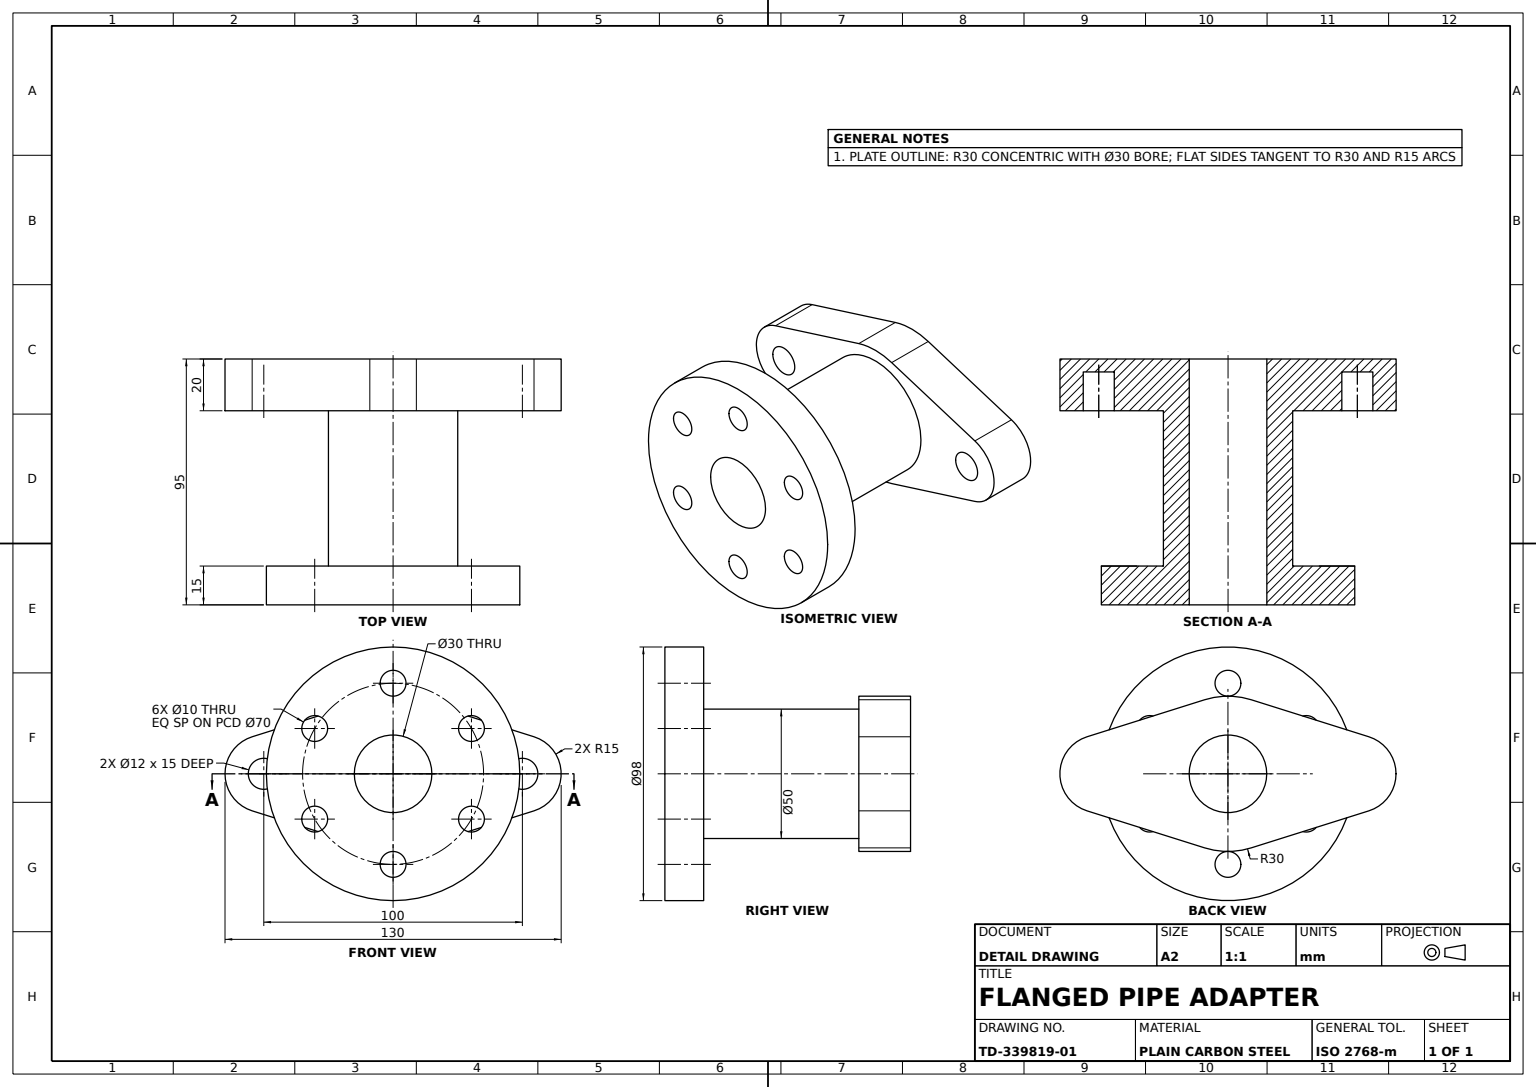
from build123d import *

# Parameters (mm, degrees)
MOUNTING_PLATE_DEPTH              = 20
HUB_SKETCH_R                      = 25
HUB_50_DEPTH                      = 60
FLANGE_SKETCH_R                   = 49
FLANGE_98_DEPTH                   = 15
FLANGE_BOLT_HOLE_SKETCH_R         = 5
FLANGE_BOLT_HOLE_10_DEPTH         = 15
BORE_SKETCH_R                     = 15
BORE_CUT_DEPTH                    = 158.006369298
FLANGE_BOLT_HOLE_PATTERN_6X_COUNT = 6
PLATE_HOLES_SKETCH_R              = 6
PLATE_HOLES_2X_12_DEPTH           = 15


with BuildPart() as part:
    # Mounting Plate Sketch → Mounting Plate (new body)
    with BuildSketch(Plane.XY):
        with BuildLine():
            Line((-4.5, 14.309088021), (41, 28.618176043))
            ThreePointArc((41, 28.618176043), (50, 30), (59, 28.618176043))
            Line((59, 28.618176043), (104.5, 14.309088021))
            ThreePointArc((104.5, 14.309088021), (115, 0), (104.5, -14.309088021))
            Line((104.5, -14.309088021), (59, -28.618176043))
            ThreePointArc((59, -28.618176043), (50, -30), (41, -28.618176043))
            Line((41, -28.618176043), (-4.5, -14.309088021))
            ThreePointArc((-4.5, -14.309088021), (-15, 0), (-4.5, 14.309088021))
        make_face()
    extrude(amount=MOUNTING_PLATE_DEPTH)

    # Hub Sketch → Hub Ø50 (add)
    with BuildSketch(Plane.XY.offset(20)):
        with Locations((50, 0)):
            Circle(HUB_SKETCH_R)
    extrude(amount=HUB_50_DEPTH)

    # Flange Sketch → Flange Ø98 (add)
    with BuildSketch(Plane.XY.offset(80)):
        with Locations((50, 0)):
            Circle(FLANGE_SKETCH_R)
    extrude(amount=FLANGE_98_DEPTH)

    # Flange Bolt Hole Sketch → Flange Bolt Hole Ø10 (cut)
    with BuildSketch(Plane.XY.offset(95)):
        with Locations((50, 35)):
            Circle(FLANGE_BOLT_HOLE_SKETCH_R)
    flange_bolt_hole_10 = extrude(amount=-FLANGE_BOLT_HOLE_10_DEPTH, mode=Mode.SUBTRACT)

    # Bore Sketch → Bore Cut (cut, through all)
    with BuildSketch(Plane.XY.offset(95)):
        with Locations((50, 0)):
            Circle(BORE_SKETCH_R)
    extrude(amount=-BORE_CUT_DEPTH, mode=Mode.SUBTRACT)

    # Flange Bolt Hole Pattern 6x: Flange Bolt Hole Ø10 ×6 about axis
    flange_bolt_hole_pattern_6x_axis = Axis((50, 0, 0), (0, 0, 1))
    for i in range(1, FLANGE_BOLT_HOLE_PATTERN_6X_COUNT):
        add(flange_bolt_hole_10.rotate(flange_bolt_hole_pattern_6x_axis, i * 360 / FLANGE_BOLT_HOLE_PATTERN_6X_COUNT), mode=Mode.SUBTRACT)

    # Plate Holes Sketch → Plate Holes 2xØ12 (cut)
    with BuildSketch(Plane.XY.offset(20)):
        Circle(PLATE_HOLES_SKETCH_R)
        with Locations((100, 0)):
            Circle(PLATE_HOLES_SKETCH_R)
    extrude(amount=-PLATE_HOLES_2X_12_DEPTH, mode=Mode.SUBTRACT)


solid = part.part
